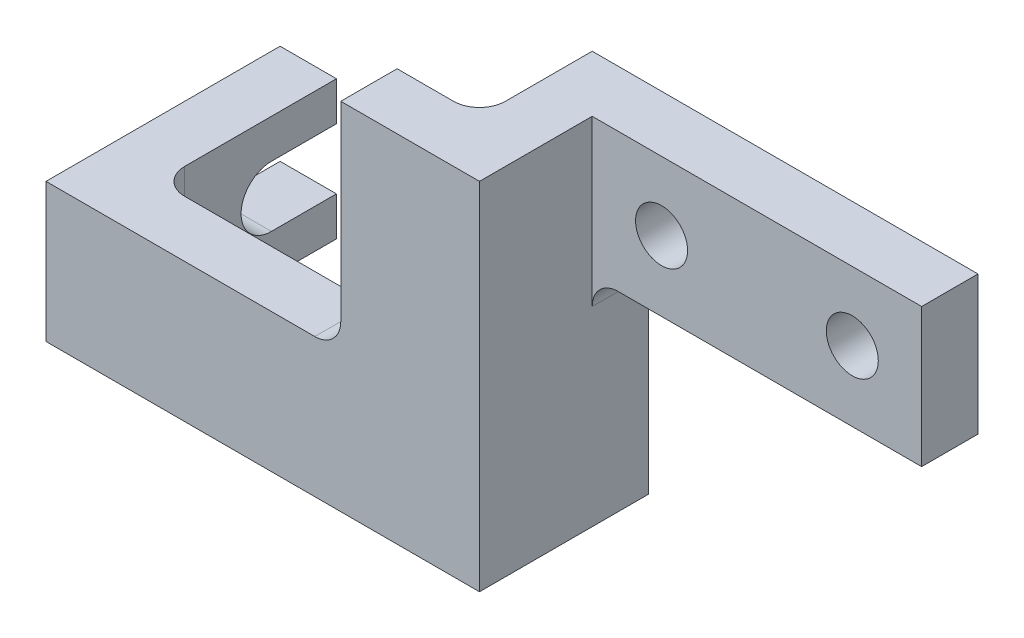
ISO-10303-21;
HEADER;
FILE_DESCRIPTION(('STEP AP214'),'2;1');
FILE_NAME('part.step','',(''),(''),'','','');
FILE_SCHEMA(('AUTOMOTIVE_DESIGN { 1 0 10303 214 1 1 1 1 }'));
ENDSEC;
DATA;
#1=APPLICATION_CONTEXT('core data for automotive mechanical design processes');
#2=APPLICATION_PROTOCOL_DEFINITION('international standard','automotive_design',2000,#1);
#3=PRODUCT_CONTEXT('',#1,'mechanical');
#4=PRODUCT('Part','Part','',(#3));
#5=PRODUCT_RELATED_PRODUCT_CATEGORY('part','',(#4));
#6=PRODUCT_DEFINITION_FORMATION('','',#4);
#7=PRODUCT_DEFINITION_CONTEXT('part definition',#1,'design');
#8=PRODUCT_DEFINITION('design','',#6,#7);
#9=PRODUCT_DEFINITION_SHAPE('','',#8);
#10=(LENGTH_UNIT() NAMED_UNIT(*) SI_UNIT(.MILLI.,.METRE.));
#11=(NAMED_UNIT(*) PLANE_ANGLE_UNIT() SI_UNIT($,.RADIAN.));
#12=(NAMED_UNIT(*) SI_UNIT($,.STERADIAN.) SOLID_ANGLE_UNIT());
#13=UNCERTAINTY_MEASURE_WITH_UNIT(LENGTH_MEASURE(1.E-05),#10,'distance_accuracy_value','');
#14=(GEOMETRIC_REPRESENTATION_CONTEXT(3) GLOBAL_UNCERTAINTY_ASSIGNED_CONTEXT((#13)) GLOBAL_UNIT_ASSIGNED_CONTEXT((#10,
#11,#12)) REPRESENTATION_CONTEXT('',''));
#15=CARTESIAN_POINT('',(0.,0.,0.));
#16=DIRECTION('',(0.,0.,1.));
#17=DIRECTION('',(1.,0.,0.));
#18=AXIS2_PLACEMENT_3D('',#15,#16,#17);
#19=CARTESIAN_POINT('',(0.,0.,-41.));
#20=DIRECTION('',(0.,0.,1.));
#21=DIRECTION('',(1.,0.,0.));
#22=AXIS2_PLACEMENT_3D('',#19,#20,#21);
#23=PLANE('',#22);
#24=DIRECTION('',(0.,-1.,0.));
#25=VECTOR('',#24,1.);
#26=CARTESIAN_POINT('',(13.,0.,-41.));
#27=LINE('',#26,#25);
#28=CARTESIAN_POINT('',(13.,32.,-41.));
#29=VERTEX_POINT('',#28);
#30=CARTESIAN_POINT('',(13.,23.,-41.));
#31=VERTEX_POINT('',#30);
#32=EDGE_CURVE('E352',#29,#31,#27,.T.);
#33=ORIENTED_EDGE('',*,*,#32,.T.);
#34=DIRECTION('',(-1.,0.,0.));
#35=VECTOR('',#34,1.);
#36=CARTESIAN_POINT('',(13.,23.,-41.));
#37=LINE('',#36,#35);
#38=CARTESIAN_POINT('',(0.,23.,-41.));
#39=VERTEX_POINT('',#38);
#40=EDGE_CURVE('E356',#31,#39,#37,.T.);
#41=ORIENTED_EDGE('',*,*,#40,.T.);
#42=DIRECTION('',(0.,1.,0.));
#43=VECTOR('',#42,1.);
#44=CARTESIAN_POINT('',(0.,32.,-41.));
#45=LINE('',#44,#43);
#46=CARTESIAN_POINT('',(0.,32.,-41.));
#47=VERTEX_POINT('',#46);
#48=EDGE_CURVE('E249',#39,#47,#45,.T.);
#49=ORIENTED_EDGE('',*,*,#48,.T.);
#50=DIRECTION('',(1.,0.,0.));
#51=VECTOR('',#50,1.);
#52=CARTESIAN_POINT('',(13.,32.,-41.));
#53=LINE('',#52,#51);
#54=EDGE_CURVE('E248',#47,#29,#53,.T.);
#55=ORIENTED_EDGE('',*,*,#54,.T.);
#56=EDGE_LOOP('',(#33,#41,#49,#55));
#57=FACE_BOUND('',#56,.T.);
#58=ADVANCED_FACE('F50',(#57),#23,.F.);
#59=CARTESIAN_POINT('',(62.,38.,0.));
#60=DIRECTION('',(0.,0.,1.));
#61=DIRECTION('',(1.,0.,0.));
#62=AXIS2_PLACEMENT_3D('',#59,#60,#61);
#63=PLANE('',#62);
#64=DIRECTION('',(0.,-1.,0.));
#65=VECTOR('',#64,1.);
#66=CARTESIAN_POINT('',(81.,82.,0.));
#67=LINE('',#66,#65);
#68=CARTESIAN_POINT('',(81.,82.,0.));
#69=VERTEX_POINT('',#68);
#70=CARTESIAN_POINT('',(81.,0.,0.));
#71=VERTEX_POINT('',#70);
#72=EDGE_CURVE('E275',#69,#71,#67,.T.);
#73=ORIENTED_EDGE('',*,*,#72,.T.);
#74=DIRECTION('',(1.,0.,0.));
#75=VECTOR('',#74,1.);
#76=CARTESIAN_POINT('',(0.,0.,0.));
#77=LINE('',#76,#75);
#78=CARTESIAN_POINT('',(19.,0.,0.));
#79=VERTEX_POINT('',#78);
#80=EDGE_CURVE('E298',#79,#71,#77,.T.);
#81=ORIENTED_EDGE('',*,*,#80,.F.);
#82=DIRECTION('',(0.,-1.,0.));
#83=VECTOR('',#82,1.);
#84=CARTESIAN_POINT('',(19.,82.,0.));
#85=LINE('',#84,#83);
#86=CARTESIAN_POINT('',(19.,32.,0.));
#87=VERTEX_POINT('',#86);
#88=EDGE_CURVE('E11',#87,#79,#85,.T.);
#89=ORIENTED_EDGE('',*,*,#88,.F.);
#90=DIRECTION('',(-1.,0.,0.));
#91=VECTOR('',#90,1.);
#92=CARTESIAN_POINT('',(62.,32.,0.));
#93=LINE('',#92,#91);
#94=CARTESIAN_POINT('',(62.,32.,0.));
#95=VERTEX_POINT('',#94);
#96=EDGE_CURVE('E296',#95,#87,#93,.T.);
#97=ORIENTED_EDGE('',*,*,#96,.F.);
#98=CARTESIAN_POINT('',(62.,38.,0.));
#99=DIRECTION('',(0.,0.,-1.));
#100=DIRECTION('',(1.,0.,0.));
#101=AXIS2_PLACEMENT_3D('',#98,#99,#100);
#102=CIRCLE('',#101,6.);
#103=CARTESIAN_POINT('',(68.,38.,0.));
#104=VERTEX_POINT('',#103);
#105=EDGE_CURVE('E317',#104,#95,#102,.T.);
#106=ORIENTED_EDGE('',*,*,#105,.F.);
#107=DIRECTION('',(0.,-1.,0.));
#108=VECTOR('',#107,1.);
#109=CARTESIAN_POINT('',(68.,82.,0.));
#110=LINE('',#109,#108);
#111=CARTESIAN_POINT('',(68.,82.,0.));
#112=VERTEX_POINT('',#111);
#113=EDGE_CURVE('E313',#112,#104,#110,.T.);
#114=ORIENTED_EDGE('',*,*,#113,.F.);
#115=DIRECTION('',(-1.,0.,0.));
#116=VECTOR('',#115,1.);
#117=CARTESIAN_POINT('',(100.,82.,0.));
#118=LINE('',#117,#116);
#119=EDGE_CURVE('E315',#69,#112,#118,.T.);
#120=ORIENTED_EDGE('',*,*,#119,.F.);
#121=EDGE_LOOP('',(#73,#81,#89,#97,#106,#114,#120));
#122=FACE_BOUND('',#121,.T.);
#123=ADVANCED_FACE('F331',(#122),#63,.F.);
#124=CARTESIAN_POINT('',(0.,32.,13.));
#125=DIRECTION('',(1.,0.,0.));
#126=DIRECTION('',(0.,0.,-1.));
#127=AXIS2_PLACEMENT_3D('',#124,#125,#126);
#128=PLANE('',#127);
#129=ORIENTED_EDGE('',*,*,#48,.F.);
#130=DIRECTION('',(0.,0.,-1.));
#131=VECTOR('',#130,1.);
#132=CARTESIAN_POINT('',(0.,23.,-26.));
#133=LINE('',#132,#131);
#134=CARTESIAN_POINT('',(0.,23.,-26.));
#135=VERTEX_POINT('',#134);
#136=EDGE_CURVE('E358',#135,#39,#133,.T.);
#137=ORIENTED_EDGE('',*,*,#136,.F.);
#138=CARTESIAN_POINT('',(0.,16.,-26.));
#139=DIRECTION('',(-1.,0.,0.));
#140=DIRECTION('',(0.,0.,1.));
#141=AXIS2_PLACEMENT_3D('',#138,#139,#140);
#142=CIRCLE('',#141,7.);
#143=CARTESIAN_POINT('',(0.,9.,-26.));
#144=VERTEX_POINT('',#143);
#145=EDGE_CURVE('E377',#144,#135,#142,.T.);
#146=ORIENTED_EDGE('',*,*,#145,.F.);
#147=DIRECTION('',(0.,0.,1.));
#148=VECTOR('',#147,1.);
#149=CARTESIAN_POINT('',(0.,9.,-41.));
#150=LINE('',#149,#148);
#151=CARTESIAN_POINT('',(0.,9.,-41.));
#152=VERTEX_POINT('',#151);
#153=EDGE_CURVE('E250',#152,#144,#150,.T.);
#154=ORIENTED_EDGE('',*,*,#153,.F.);
#155=CARTESIAN_POINT('',(0.,0.,-41.));
#156=VERTEX_POINT('',#155);
#157=EDGE_CURVE('E242',#156,#152,#45,.T.);
#158=ORIENTED_EDGE('',*,*,#157,.F.);
#159=DIRECTION('',(0.,0.,-1.));
#160=VECTOR('',#159,1.);
#161=CARTESIAN_POINT('',(0.,0.,13.));
#162=LINE('',#161,#160);
#163=CARTESIAN_POINT('',(0.,0.,13.));
#164=VERTEX_POINT('',#163);
#165=EDGE_CURVE('E54',#164,#156,#162,.T.);
#166=ORIENTED_EDGE('',*,*,#165,.F.);
#167=DIRECTION('',(0.,-1.,0.));
#168=VECTOR('',#167,1.);
#169=CARTESIAN_POINT('',(0.,32.,13.));
#170=LINE('',#169,#168);
#171=CARTESIAN_POINT('',(0.,32.,13.));
#172=VERTEX_POINT('',#171);
#173=EDGE_CURVE('E241',#172,#164,#170,.T.);
#174=ORIENTED_EDGE('',*,*,#173,.F.);
#175=DIRECTION('',(0.,0.,-1.));
#176=VECTOR('',#175,1.);
#177=CARTESIAN_POINT('',(0.,32.,13.));
#178=LINE('',#177,#176);
#179=EDGE_CURVE('E307',#172,#47,#178,.T.);
#180=ORIENTED_EDGE('',*,*,#179,.T.);
#181=EDGE_LOOP('',(#129,#137,#146,#154,#158,#166,#174,#180));
#182=FACE_BOUND('',#181,.T.);
#183=ADVANCED_FACE('F47',(#182),#128,.F.);
#184=CARTESIAN_POINT('',(0.,0.,13.));
#185=DIRECTION('',(0.,1.,0.));
#186=DIRECTION('',(0.,0.,1.));
#187=AXIS2_PLACEMENT_3D('',#184,#185,#186);
#188=PLANE('',#187);
#189=ORIENTED_EDGE('',*,*,#165,.T.);
#190=DIRECTION('',(-1.,0.,0.));
#191=VECTOR('',#190,1.);
#192=CARTESIAN_POINT('',(0.,0.,-41.));
#193=LINE('',#192,#191);
#194=CARTESIAN_POINT('',(13.,0.,-41.));
#195=VERTEX_POINT('',#194);
#196=EDGE_CURVE('E233',#195,#156,#193,.T.);
#197=ORIENTED_EDGE('',*,*,#196,.F.);
#198=DIRECTION('',(0.,0.,1.));
#199=VECTOR('',#198,1.);
#200=CARTESIAN_POINT('',(13.,0.,0.));
#201=LINE('',#200,#199);
#202=CARTESIAN_POINT('',(13.,0.,-6.00000000000004));
#203=VERTEX_POINT('',#202);
#204=EDGE_CURVE('E293',#195,#203,#201,.T.);
#205=ORIENTED_EDGE('',*,*,#204,.T.);
#206=CARTESIAN_POINT('',(19.,0.,-6.));
#207=DIRECTION('',(0.,-1.,0.));
#208=DIRECTION('',(0.,0.,-1.));
#209=AXIS2_PLACEMENT_3D('',#206,#207,#208);
#210=CIRCLE('',#209,6.);
#211=EDGE_CURVE('E281',#79,#203,#210,.T.);
#212=ORIENTED_EDGE('',*,*,#211,.F.);
#213=ORIENTED_EDGE('',*,*,#80,.T.);
#214=CARTESIAN_POINT('',(81.,0.,-6.));
#215=DIRECTION('',(0.,-1.,0.));
#216=DIRECTION('',(0.,0.,-1.));
#217=AXIS2_PLACEMENT_3D('',#214,#215,#216);
#218=CIRCLE('',#217,6.);
#219=CARTESIAN_POINT('',(87.,0.,-6.00000000000004));
#220=VERTEX_POINT('',#219);
#221=EDGE_CURVE('E261',#71,#220,#218,.F.);
#222=ORIENTED_EDGE('',*,*,#221,.T.);
#223=DIRECTION('',(0.,0.,-1.));
#224=VECTOR('',#223,1.);
#225=CARTESIAN_POINT('',(87.,0.,0.));
#226=LINE('',#225,#224);
#227=CARTESIAN_POINT('',(87.,0.,-26.));
#228=VERTEX_POINT('',#227);
#229=EDGE_CURVE('E273',#220,#228,#226,.T.);
#230=ORIENTED_EDGE('',*,*,#229,.T.);
#231=DIRECTION('',(1.,0.,0.));
#232=VECTOR('',#231,1.);
#233=CARTESIAN_POINT('',(0.,0.,-26.));
#234=LINE('',#233,#232);
#235=CARTESIAN_POINT('',(100.,0.,-26.));
#236=VERTEX_POINT('',#235);
#237=EDGE_CURVE('E270',#228,#236,#234,.T.);
#238=ORIENTED_EDGE('',*,*,#237,.T.);
#239=DIRECTION('',(0.,0.,-1.));
#240=VECTOR('',#239,1.);
#241=CARTESIAN_POINT('',(100.,0.,13.));
#242=LINE('',#241,#240);
#243=CARTESIAN_POINT('',(100.,0.,13.));
#244=VERTEX_POINT('',#243);
#245=EDGE_CURVE('E216',#244,#236,#242,.T.);
#246=ORIENTED_EDGE('',*,*,#245,.F.);
#247=DIRECTION('',(1.,0.,0.));
#248=VECTOR('',#247,1.);
#249=CARTESIAN_POINT('',(0.,0.,13.));
#250=LINE('',#249,#248);
#251=EDGE_CURVE('E234',#164,#244,#250,.T.);
#252=ORIENTED_EDGE('',*,*,#251,.F.);
#253=EDGE_LOOP('',(#189,#197,#205,#212,#213,#222,#230,#238,#246,#252));
#254=FACE_BOUND('',#253,.T.);
#255=ADVANCED_FACE('F229',(#254),#188,.F.);
#256=CARTESIAN_POINT('',(100.,0.,13.));
#257=DIRECTION('',(-1.,0.,0.));
#258=DIRECTION('',(0.,0.,1.));
#259=AXIS2_PLACEMENT_3D('',#256,#257,#258);
#260=PLANE('',#259);
#261=DIRECTION('',(0.,-1.,0.));
#262=VECTOR('',#261,1.);
#263=CARTESIAN_POINT('',(100.,82.,-26.));
#264=LINE('',#263,#262);
#265=CARTESIAN_POINT('',(100.,44.,-26.));
#266=VERTEX_POINT('',#265);
#267=EDGE_CURVE('E278',#266,#236,#264,.T.);
#268=ORIENTED_EDGE('',*,*,#267,.F.);
#269=DIRECTION('',(0.,0.,-1.));
#270=VECTOR('',#269,1.);
#271=CARTESIAN_POINT('',(100.,44.,-13.));
#272=LINE('',#271,#270);
#273=CARTESIAN_POINT('',(100.,44.,-13.));
#274=VERTEX_POINT('',#273);
#275=EDGE_CURVE('E215',#274,#266,#272,.T.);
#276=ORIENTED_EDGE('',*,*,#275,.F.);
#277=DIRECTION('',(0.,1.,0.));
#278=VECTOR('',#277,1.);
#279=CARTESIAN_POINT('',(100.,82.,-13.));
#280=LINE('',#279,#278);
#281=CARTESIAN_POINT('',(100.,82.,-13.));
#282=VERTEX_POINT('',#281);
#283=EDGE_CURVE('E193',#274,#282,#280,.T.);
#284=ORIENTED_EDGE('',*,*,#283,.T.);
#285=DIRECTION('',(0.,0.,-1.));
#286=VECTOR('',#285,1.);
#287=CARTESIAN_POINT('',(100.,82.,13.));
#288=LINE('',#287,#286);
#289=CARTESIAN_POINT('',(100.,82.,13.));
#290=VERTEX_POINT('',#289);
#291=EDGE_CURVE('E208',#290,#282,#288,.T.);
#292=ORIENTED_EDGE('',*,*,#291,.F.);
#293=DIRECTION('',(0.,1.,0.));
#294=VECTOR('',#293,1.);
#295=CARTESIAN_POINT('',(100.,0.,13.));
#296=LINE('',#295,#294);
#297=EDGE_CURVE('E297',#244,#290,#296,.T.);
#298=ORIENTED_EDGE('',*,*,#297,.F.);
#299=ORIENTED_EDGE('',*,*,#245,.T.);
#300=EDGE_LOOP('',(#268,#276,#284,#292,#298,#299));
#301=FACE_BOUND('',#300,.T.);
#302=ADVANCED_FACE('F206',(#301),#260,.F.);
#303=CARTESIAN_POINT('',(100.,82.,13.));
#304=DIRECTION('',(0.,-1.,0.));
#305=DIRECTION('',(0.,0.,-1.));
#306=AXIS2_PLACEMENT_3D('',#303,#304,#305);
#307=PLANE('',#306);
#308=ORIENTED_EDGE('',*,*,#291,.T.);
#309=DIRECTION('',(1.,0.,0.));
#310=VECTOR('',#309,1.);
#311=CARTESIAN_POINT('',(100.,82.,-13.));
#312=LINE('',#311,#310);
#313=CARTESIAN_POINT('',(176.,82.,-13.));
#314=VERTEX_POINT('',#313);
#315=EDGE_CURVE('E192',#282,#314,#312,.T.);
#316=ORIENTED_EDGE('',*,*,#315,.T.);
#317=DIRECTION('',(0.,0.,-1.));
#318=VECTOR('',#317,1.);
#319=CARTESIAN_POINT('',(176.,82.,-13.));
#320=LINE('',#319,#318);
#321=CARTESIAN_POINT('',(176.,82.,-26.));
#322=VERTEX_POINT('',#321);
#323=EDGE_CURVE('E379',#314,#322,#320,.T.);
#324=ORIENTED_EDGE('',*,*,#323,.T.);
#325=DIRECTION('',(1.,0.,0.));
#326=VECTOR('',#325,1.);
#327=CARTESIAN_POINT('',(0.,82.,-26.));
#328=LINE('',#327,#326);
#329=CARTESIAN_POINT('',(87.,82.,-26.));
#330=VERTEX_POINT('',#329);
#331=EDGE_CURVE('E268',#330,#322,#328,.T.);
#332=ORIENTED_EDGE('',*,*,#331,.F.);
#333=DIRECTION('',(0.,0.,-1.));
#334=VECTOR('',#333,1.);
#335=CARTESIAN_POINT('',(87.,82.,0.));
#336=LINE('',#335,#334);
#337=CARTESIAN_POINT('',(87.,82.,-6.00000000000004));
#338=VERTEX_POINT('',#337);
#339=EDGE_CURVE('E267',#338,#330,#336,.T.);
#340=ORIENTED_EDGE('',*,*,#339,.F.);
#341=CARTESIAN_POINT('',(81.,82.,-6.));
#342=DIRECTION('',(0.,-1.,0.));
#343=DIRECTION('',(0.,0.,-1.));
#344=AXIS2_PLACEMENT_3D('',#341,#342,#343);
#345=CIRCLE('',#344,6.);
#346=EDGE_CURVE('E265',#69,#338,#345,.F.);
#347=ORIENTED_EDGE('',*,*,#346,.F.);
#348=ORIENTED_EDGE('',*,*,#119,.T.);
#349=DIRECTION('',(0.,0.,-1.));
#350=VECTOR('',#349,1.);
#351=CARTESIAN_POINT('',(68.,82.,13.));
#352=LINE('',#351,#350);
#353=CARTESIAN_POINT('',(68.,82.,13.));
#354=VERTEX_POINT('',#353);
#355=EDGE_CURVE('E220',#354,#112,#352,.T.);
#356=ORIENTED_EDGE('',*,*,#355,.F.);
#357=DIRECTION('',(-1.,0.,0.));
#358=VECTOR('',#357,1.);
#359=CARTESIAN_POINT('',(100.,82.,13.));
#360=LINE('',#359,#358);
#361=EDGE_CURVE('E219',#290,#354,#360,.T.);
#362=ORIENTED_EDGE('',*,*,#361,.F.);
#363=EDGE_LOOP('',(#308,#316,#324,#332,#340,#347,#348,#356,#362));
#364=FACE_BOUND('',#363,.T.);
#365=ADVANCED_FACE('F211',(#364),#307,.F.);
#366=CARTESIAN_POINT('',(68.,82.,13.));
#367=DIRECTION('',(1.,0.,0.));
#368=DIRECTION('',(0.,0.,-1.));
#369=AXIS2_PLACEMENT_3D('',#366,#367,#368);
#370=PLANE('',#369);
#371=ORIENTED_EDGE('',*,*,#113,.T.);
#372=DIRECTION('',(0.,0.,-1.));
#373=VECTOR('',#372,1.);
#374=CARTESIAN_POINT('',(68.,38.,13.));
#375=LINE('',#374,#373);
#376=CARTESIAN_POINT('',(68.,38.,13.));
#377=VERTEX_POINT('',#376);
#378=EDGE_CURVE('E224',#377,#104,#375,.T.);
#379=ORIENTED_EDGE('',*,*,#378,.F.);
#380=DIRECTION('',(0.,-1.,0.));
#381=VECTOR('',#380,1.);
#382=CARTESIAN_POINT('',(68.,82.,13.));
#383=LINE('',#382,#381);
#384=EDGE_CURVE('E303',#354,#377,#383,.T.);
#385=ORIENTED_EDGE('',*,*,#384,.F.);
#386=ORIENTED_EDGE('',*,*,#355,.T.);
#387=EDGE_LOOP('',(#371,#379,#385,#386));
#388=FACE_BOUND('',#387,.T.);
#389=ADVANCED_FACE('F441',(#388),#370,.F.);
#390=CARTESIAN_POINT('',(62.,38.,13.));
#391=DIRECTION('',(0.,0.,-1.));
#392=DIRECTION('',(-1.,0.,0.));
#393=AXIS2_PLACEMENT_3D('',#390,#391,#392);
#394=CYLINDRICAL_SURFACE('',#393,6.);
#395=ORIENTED_EDGE('',*,*,#105,.T.);
#396=DIRECTION('',(0.,0.,-1.));
#397=VECTOR('',#396,1.);
#398=CARTESIAN_POINT('',(62.,32.,13.));
#399=LINE('',#398,#397);
#400=CARTESIAN_POINT('',(62.,32.,13.));
#401=VERTEX_POINT('',#400);
#402=EDGE_CURVE('E318',#401,#95,#399,.T.);
#403=ORIENTED_EDGE('',*,*,#402,.F.);
#404=CARTESIAN_POINT('',(62.,38.,13.));
#405=DIRECTION('',(0.,0.,-1.));
#406=DIRECTION('',(1.,0.,0.));
#407=AXIS2_PLACEMENT_3D('',#404,#405,#406);
#408=CIRCLE('',#407,6.);
#409=EDGE_CURVE('E304',#377,#401,#408,.T.);
#410=ORIENTED_EDGE('',*,*,#409,.F.);
#411=ORIENTED_EDGE('',*,*,#378,.T.);
#412=EDGE_LOOP('',(#395,#403,#410,#411));
#413=FACE_BOUND('',#412,.T.);
#414=ADVANCED_FACE('F326',(#413),#394,.F.);
#415=CARTESIAN_POINT('',(62.,32.,13.));
#416=DIRECTION('',(0.,-1.,0.));
#417=DIRECTION('',(0.,0.,-1.));
#418=AXIS2_PLACEMENT_3D('',#415,#416,#417);
#419=PLANE('',#418);
#420=DIRECTION('',(0.,0.,-1.));
#421=VECTOR('',#420,1.);
#422=CARTESIAN_POINT('',(13.,32.,0.));
#423=LINE('',#422,#421);
#424=CARTESIAN_POINT('',(13.,32.,-6.00000000000004));
#425=VERTEX_POINT('',#424);
#426=EDGE_CURVE('E255',#425,#29,#423,.T.);
#427=ORIENTED_EDGE('',*,*,#426,.T.);
#428=ORIENTED_EDGE('',*,*,#54,.F.);
#429=ORIENTED_EDGE('',*,*,#179,.F.);
#430=DIRECTION('',(-1.,0.,0.));
#431=VECTOR('',#430,1.);
#432=CARTESIAN_POINT('',(62.,32.,13.));
#433=LINE('',#432,#431);
#434=EDGE_CURVE('E310',#401,#172,#433,.T.);
#435=ORIENTED_EDGE('',*,*,#434,.F.);
#436=ORIENTED_EDGE('',*,*,#402,.T.);
#437=ORIENTED_EDGE('',*,*,#96,.T.);
#438=CARTESIAN_POINT('',(19.,32.,-6.));
#439=DIRECTION('',(0.,-1.,0.));
#440=DIRECTION('',(0.,0.,-1.));
#441=AXIS2_PLACEMENT_3D('',#438,#439,#440);
#442=CIRCLE('',#441,6.);
#443=EDGE_CURVE('E256',#425,#87,#442,.F.);
#444=ORIENTED_EDGE('',*,*,#443,.F.);
#445=EDGE_LOOP('',(#427,#428,#429,#435,#436,#437,#444));
#446=FACE_BOUND('',#445,.T.);
#447=ADVANCED_FACE('F339',(#446),#419,.F.);
#448=CARTESIAN_POINT('',(62.,38.,13.));
#449=DIRECTION('',(0.,0.,1.));
#450=DIRECTION('',(1.,0.,0.));
#451=AXIS2_PLACEMENT_3D('',#448,#449,#450);
#452=PLANE('',#451);
#453=ORIENTED_EDGE('',*,*,#173,.T.);
#454=ORIENTED_EDGE('',*,*,#251,.T.);
#455=ORIENTED_EDGE('',*,*,#297,.T.);
#456=ORIENTED_EDGE('',*,*,#361,.T.);
#457=ORIENTED_EDGE('',*,*,#384,.T.);
#458=ORIENTED_EDGE('',*,*,#409,.T.);
#459=ORIENTED_EDGE('',*,*,#434,.T.);
#460=EDGE_LOOP('',(#453,#454,#455,#456,#457,#458,#459));
#461=FACE_BOUND('',#460,.T.);
#462=ADVANCED_FACE('F433',(#461),#452,.T.);
#463=CARTESIAN_POINT('',(19.,82.,-6.));
#464=DIRECTION('',(0.,-1.,0.));
#465=DIRECTION('',(0.,0.,-1.));
#466=AXIS2_PLACEMENT_3D('',#463,#464,#465);
#467=CYLINDRICAL_SURFACE('',#466,6.);
#468=DIRECTION('',(0.,-1.,0.));
#469=VECTOR('',#468,1.);
#470=CARTESIAN_POINT('',(13.,82.,-6.00000000000004));
#471=LINE('',#470,#469);
#472=EDGE_CURVE('E291',#425,#203,#471,.T.);
#473=ORIENTED_EDGE('',*,*,#472,.F.);
#474=ORIENTED_EDGE('',*,*,#443,.T.);
#475=ORIENTED_EDGE('',*,*,#88,.T.);
#476=ORIENTED_EDGE('',*,*,#211,.T.);
#477=EDGE_LOOP('',(#473,#474,#475,#476));
#478=FACE_BOUND('',#477,.T.);
#479=ADVANCED_FACE('F341',(#478),#467,.F.);
#480=CARTESIAN_POINT('',(13.,82.,0.));
#481=DIRECTION('',(1.,0.,0.));
#482=DIRECTION('',(0.,0.,-1.));
#483=AXIS2_PLACEMENT_3D('',#480,#481,#482);
#484=PLANE('',#483);
#485=DIRECTION('',(0.,0.,-1.));
#486=VECTOR('',#485,1.);
#487=CARTESIAN_POINT('',(13.,23.,-26.));
#488=LINE('',#487,#486);
#489=CARTESIAN_POINT('',(13.,23.,-26.));
#490=VERTEX_POINT('',#489);
#491=EDGE_CURVE('E371',#490,#31,#488,.T.);
#492=ORIENTED_EDGE('',*,*,#491,.T.);
#493=ORIENTED_EDGE('',*,*,#32,.F.);
#494=ORIENTED_EDGE('',*,*,#426,.F.);
#495=ORIENTED_EDGE('',*,*,#472,.T.);
#496=ORIENTED_EDGE('',*,*,#204,.F.);
#497=CARTESIAN_POINT('',(13.,9.,-41.));
#498=VERTEX_POINT('',#497);
#499=EDGE_CURVE('E363',#498,#195,#27,.T.);
#500=ORIENTED_EDGE('',*,*,#499,.F.);
#501=DIRECTION('',(0.,0.,1.));
#502=VECTOR('',#501,1.);
#503=CARTESIAN_POINT('',(13.,9.,-41.));
#504=LINE('',#503,#502);
#505=CARTESIAN_POINT('',(13.,9.,-26.));
#506=VERTEX_POINT('',#505);
#507=EDGE_CURVE('E67',#498,#506,#504,.T.);
#508=ORIENTED_EDGE('',*,*,#507,.T.);
#509=CARTESIAN_POINT('',(13.,16.,-26.));
#510=DIRECTION('',(-1.,0.,0.));
#511=DIRECTION('',(0.,0.,1.));
#512=AXIS2_PLACEMENT_3D('',#509,#510,#511);
#513=CIRCLE('',#512,7.);
#514=EDGE_CURVE('E374',#506,#490,#513,.T.);
#515=ORIENTED_EDGE('',*,*,#514,.T.);
#516=EDGE_LOOP('',(#492,#493,#494,#495,#496,#500,#508,#515));
#517=FACE_BOUND('',#516,.T.);
#518=ADVANCED_FACE('F346',(#517),#484,.T.);
#519=CARTESIAN_POINT('',(0.,82.,-26.));
#520=DIRECTION('',(0.,0.,-1.));
#521=DIRECTION('',(-1.,0.,0.));
#522=AXIS2_PLACEMENT_3D('',#519,#520,#521);
#523=PLANE('',#522);
#524=CARTESIAN_POINT('',(116.,66.1568766824244,-26.));
#525=DIRECTION('',(0.,0.,1.));
#526=DIRECTION('',(1.,0.,0.));
#527=AXIS2_PLACEMENT_3D('',#524,#525,#526);
#528=CIRCLE('',#527,5.99999999999999);
#529=CARTESIAN_POINT('',(122.,66.1568766824244,-26.));
#530=VERTEX_POINT('',#529);
#531=EDGE_CURVE('E706',#530,#530,#528,.T.);
#532=ORIENTED_EDGE('',*,*,#531,.T.);
#533=EDGE_LOOP('',(#532));
#534=FACE_BOUND('',#533,.T.);
#535=CARTESIAN_POINT('',(160.,66.1568766824244,-26.));
#536=DIRECTION('',(0.,0.,1.));
#537=DIRECTION('',(1.,0.,0.));
#538=AXIS2_PLACEMENT_3D('',#535,#536,#537);
#539=CIRCLE('',#538,5.99999999999999);
#540=CARTESIAN_POINT('',(166.,66.1568766824244,-26.));
#541=VERTEX_POINT('',#540);
#542=EDGE_CURVE('E715',#541,#541,#539,.T.);
#543=ORIENTED_EDGE('',*,*,#542,.T.);
#544=EDGE_LOOP('',(#543));
#545=FACE_BOUND('',#544,.T.);
#546=ORIENTED_EDGE('',*,*,#237,.F.);
#547=DIRECTION('',(0.,-1.,0.));
#548=VECTOR('',#547,1.);
#549=CARTESIAN_POINT('',(87.,82.,-26.));
#550=LINE('',#549,#548);
#551=EDGE_CURVE('E285',#330,#228,#550,.T.);
#552=ORIENTED_EDGE('',*,*,#551,.F.);
#553=ORIENTED_EDGE('',*,*,#331,.T.);
#554=DIRECTION('',(0.,-1.,0.));
#555=VECTOR('',#554,1.);
#556=CARTESIAN_POINT('',(176.,82.,-26.));
#557=LINE('',#556,#555);
#558=CARTESIAN_POINT('',(176.,50.,-26.));
#559=VERTEX_POINT('',#558);
#560=EDGE_CURVE('E717',#322,#559,#557,.T.);
#561=ORIENTED_EDGE('',*,*,#560,.T.);
#562=DIRECTION('',(-1.,0.,0.));
#563=VECTOR('',#562,1.);
#564=CARTESIAN_POINT('',(176.,50.,-26.));
#565=LINE('',#564,#563);
#566=CARTESIAN_POINT('',(106.,50.,-26.));
#567=VERTEX_POINT('',#566);
#568=EDGE_CURVE('E725',#559,#567,#565,.T.);
#569=ORIENTED_EDGE('',*,*,#568,.T.);
#570=CARTESIAN_POINT('',(106.,44.,-26.));
#571=DIRECTION('',(0.,0.,1.));
#572=DIRECTION('',(1.,0.,0.));
#573=AXIS2_PLACEMENT_3D('',#570,#571,#572);
#574=CIRCLE('',#573,6.);
#575=EDGE_CURVE('E65',#567,#266,#574,.T.);
#576=ORIENTED_EDGE('',*,*,#575,.T.);
#577=ORIENTED_EDGE('',*,*,#267,.T.);
#578=EDGE_LOOP('',(#546,#552,#553,#561,#569,#576,#577));
#579=FACE_BOUND('',#578,.T.);
#580=ADVANCED_FACE('F428',(#534,#545,#579),#523,.T.);
#581=CARTESIAN_POINT('',(87.,82.,0.));
#582=DIRECTION('',(-1.,0.,0.));
#583=DIRECTION('',(0.,0.,1.));
#584=AXIS2_PLACEMENT_3D('',#581,#582,#583);
#585=PLANE('',#584);
#586=ORIENTED_EDGE('',*,*,#229,.F.);
#587=DIRECTION('',(0.,-1.,0.));
#588=VECTOR('',#587,1.);
#589=CARTESIAN_POINT('',(87.,82.,-6.00000000000004));
#590=LINE('',#589,#588);
#591=EDGE_CURVE('E282',#338,#220,#590,.T.);
#592=ORIENTED_EDGE('',*,*,#591,.F.);
#593=ORIENTED_EDGE('',*,*,#339,.T.);
#594=ORIENTED_EDGE('',*,*,#551,.T.);
#595=EDGE_LOOP('',(#586,#592,#593,#594));
#596=FACE_BOUND('',#595,.T.);
#597=ADVANCED_FACE('F416',(#596),#585,.T.);
#598=CARTESIAN_POINT('',(81.,82.,-6.));
#599=DIRECTION('',(0.,-1.,0.));
#600=DIRECTION('',(0.,0.,-1.));
#601=AXIS2_PLACEMENT_3D('',#598,#599,#600);
#602=CYLINDRICAL_SURFACE('',#601,6.);
#603=ORIENTED_EDGE('',*,*,#221,.F.);
#604=ORIENTED_EDGE('',*,*,#72,.F.);
#605=ORIENTED_EDGE('',*,*,#346,.T.);
#606=ORIENTED_EDGE('',*,*,#591,.T.);
#607=EDGE_LOOP('',(#603,#604,#605,#606));
#608=FACE_BOUND('',#607,.T.);
#609=ADVANCED_FACE('F414',(#608),#602,.F.);
#610=ORIENTED_EDGE('',*,*,#157,.T.);
#611=DIRECTION('',(-1.,0.,0.));
#612=VECTOR('',#611,1.);
#613=CARTESIAN_POINT('',(13.,9.,-41.));
#614=LINE('',#613,#612);
#615=EDGE_CURVE('E369',#498,#152,#614,.T.);
#616=ORIENTED_EDGE('',*,*,#615,.F.);
#617=ORIENTED_EDGE('',*,*,#499,.T.);
#618=ORIENTED_EDGE('',*,*,#196,.T.);
#619=EDGE_LOOP('',(#610,#616,#617,#618));
#620=FACE_BOUND('',#619,.T.);
#621=ADVANCED_FACE('F375',(#620),#23,.F.);
#622=CARTESIAN_POINT('',(13.,23.,-26.));
#623=DIRECTION('',(0.,1.,0.));
#624=DIRECTION('',(0.,0.,1.));
#625=AXIS2_PLACEMENT_3D('',#622,#623,#624);
#626=PLANE('',#625);
#627=ORIENTED_EDGE('',*,*,#136,.T.);
#628=ORIENTED_EDGE('',*,*,#40,.F.);
#629=ORIENTED_EDGE('',*,*,#491,.F.);
#630=DIRECTION('',(-1.,0.,0.));
#631=VECTOR('',#630,1.);
#632=CARTESIAN_POINT('',(13.,23.,-26.));
#633=LINE('',#632,#631);
#634=EDGE_CURVE('E365',#490,#135,#633,.T.);
#635=ORIENTED_EDGE('',*,*,#634,.T.);
#636=EDGE_LOOP('',(#627,#628,#629,#635));
#637=FACE_BOUND('',#636,.T.);
#638=ADVANCED_FACE('F396',(#637),#626,.F.);
#639=CARTESIAN_POINT('',(13.,16.,-26.));
#640=DIRECTION('',(-1.,0.,0.));
#641=DIRECTION('',(0.,0.,1.));
#642=AXIS2_PLACEMENT_3D('',#639,#640,#641);
#643=CYLINDRICAL_SURFACE('',#642,7.);
#644=ORIENTED_EDGE('',*,*,#145,.T.);
#645=ORIENTED_EDGE('',*,*,#634,.F.);
#646=ORIENTED_EDGE('',*,*,#514,.F.);
#647=DIRECTION('',(-1.,0.,0.));
#648=VECTOR('',#647,1.);
#649=CARTESIAN_POINT('',(13.,9.,-26.));
#650=LINE('',#649,#648);
#651=EDGE_CURVE('E364',#506,#144,#650,.T.);
#652=ORIENTED_EDGE('',*,*,#651,.T.);
#653=EDGE_LOOP('',(#644,#645,#646,#652));
#654=FACE_BOUND('',#653,.T.);
#655=ADVANCED_FACE('F387',(#654),#643,.F.);
#656=CARTESIAN_POINT('',(13.,9.,-41.));
#657=DIRECTION('',(0.,-1.,0.));
#658=DIRECTION('',(0.,0.,-1.));
#659=AXIS2_PLACEMENT_3D('',#656,#657,#658);
#660=PLANE('',#659);
#661=ORIENTED_EDGE('',*,*,#153,.T.);
#662=ORIENTED_EDGE('',*,*,#651,.F.);
#663=ORIENTED_EDGE('',*,*,#507,.F.);
#664=ORIENTED_EDGE('',*,*,#615,.T.);
#665=EDGE_LOOP('',(#661,#662,#663,#664));
#666=FACE_BOUND('',#665,.T.);
#667=ADVANCED_FACE('F390',(#666),#660,.F.);
#668=CARTESIAN_POINT('',(106.,44.,-13.));
#669=DIRECTION('',(0.,0.,-1.));
#670=DIRECTION('',(-1.,0.,0.));
#671=AXIS2_PLACEMENT_3D('',#668,#669,#670);
#672=CYLINDRICAL_SURFACE('',#671,6.);
#673=ORIENTED_EDGE('',*,*,#575,.F.);
#674=DIRECTION('',(0.,0.,-1.));
#675=VECTOR('',#674,1.);
#676=CARTESIAN_POINT('',(106.,50.,-13.));
#677=LINE('',#676,#675);
#678=CARTESIAN_POINT('',(106.,50.,-13.));
#679=VERTEX_POINT('',#678);
#680=EDGE_CURVE('E734',#679,#567,#677,.T.);
#681=ORIENTED_EDGE('',*,*,#680,.F.);
#682=CARTESIAN_POINT('',(106.,44.,-13.));
#683=DIRECTION('',(0.,0.,1.));
#684=DIRECTION('',(1.,0.,0.));
#685=AXIS2_PLACEMENT_3D('',#682,#683,#684);
#686=CIRCLE('',#685,6.);
#687=EDGE_CURVE('E726',#679,#274,#686,.T.);
#688=ORIENTED_EDGE('',*,*,#687,.T.);
#689=ORIENTED_EDGE('',*,*,#275,.T.);
#690=EDGE_LOOP('',(#673,#681,#688,#689));
#691=FACE_BOUND('',#690,.T.);
#692=ADVANCED_FACE('F386',(#691),#672,.F.);
#693=CARTESIAN_POINT('',(176.,50.,-13.));
#694=DIRECTION('',(0.,-1.,0.));
#695=DIRECTION('',(0.,0.,-1.));
#696=AXIS2_PLACEMENT_3D('',#693,#694,#695);
#697=PLANE('',#696);
#698=ORIENTED_EDGE('',*,*,#568,.F.);
#699=DIRECTION('',(0.,0.,-1.));
#700=VECTOR('',#699,1.);
#701=CARTESIAN_POINT('',(176.,50.,-13.));
#702=LINE('',#701,#700);
#703=CARTESIAN_POINT('',(176.,50.,-13.));
#704=VERTEX_POINT('',#703);
#705=EDGE_CURVE('E731',#704,#559,#702,.T.);
#706=ORIENTED_EDGE('',*,*,#705,.F.);
#707=DIRECTION('',(-1.,0.,0.));
#708=VECTOR('',#707,1.);
#709=CARTESIAN_POINT('',(176.,50.,-13.));
#710=LINE('',#709,#708);
#711=EDGE_CURVE('E733',#704,#679,#710,.T.);
#712=ORIENTED_EDGE('',*,*,#711,.T.);
#713=ORIENTED_EDGE('',*,*,#680,.T.);
#714=EDGE_LOOP('',(#698,#706,#712,#713));
#715=FACE_BOUND('',#714,.T.);
#716=ADVANCED_FACE('F397',(#715),#697,.T.);
#717=CARTESIAN_POINT('',(176.,82.,-13.));
#718=DIRECTION('',(1.,0.,0.));
#719=DIRECTION('',(0.,0.,-1.));
#720=AXIS2_PLACEMENT_3D('',#717,#718,#719);
#721=PLANE('',#720);
#722=ORIENTED_EDGE('',*,*,#560,.F.);
#723=ORIENTED_EDGE('',*,*,#323,.F.);
#724=DIRECTION('',(0.,-1.,0.));
#725=VECTOR('',#724,1.);
#726=CARTESIAN_POINT('',(176.,82.,-13.));
#727=LINE('',#726,#725);
#728=EDGE_CURVE('E198',#314,#704,#727,.T.);
#729=ORIENTED_EDGE('',*,*,#728,.T.);
#730=ORIENTED_EDGE('',*,*,#705,.T.);
#731=EDGE_LOOP('',(#722,#723,#729,#730));
#732=FACE_BOUND('',#731,.T.);
#733=ADVANCED_FACE('F547',(#732),#721,.T.);
#734=CARTESIAN_POINT('',(106.,44.,-13.));
#735=DIRECTION('',(0.,0.,1.));
#736=DIRECTION('',(1.,0.,0.));
#737=AXIS2_PLACEMENT_3D('',#734,#735,#736);
#738=PLANE('',#737);
#739=CARTESIAN_POINT('',(116.,66.1568766824244,-13.));
#740=DIRECTION('',(0.,0.,1.));
#741=DIRECTION('',(1.,0.,0.));
#742=AXIS2_PLACEMENT_3D('',#739,#740,#741);
#743=CIRCLE('',#742,5.99999999999999);
#744=CARTESIAN_POINT('',(122.,66.1568766824244,-13.));
#745=VERTEX_POINT('',#744);
#746=EDGE_CURVE('E723',#745,#745,#743,.T.);
#747=ORIENTED_EDGE('',*,*,#746,.F.);
#748=EDGE_LOOP('',(#747));
#749=FACE_BOUND('',#748,.T.);
#750=CARTESIAN_POINT('',(160.,66.1568766824244,-13.));
#751=DIRECTION('',(0.,0.,1.));
#752=DIRECTION('',(1.,0.,0.));
#753=AXIS2_PLACEMENT_3D('',#750,#751,#752);
#754=CIRCLE('',#753,5.99999999999999);
#755=CARTESIAN_POINT('',(166.,66.1568766824244,-13.));
#756=VERTEX_POINT('',#755);
#757=EDGE_CURVE('E738',#756,#756,#754,.T.);
#758=ORIENTED_EDGE('',*,*,#757,.F.);
#759=EDGE_LOOP('',(#758));
#760=FACE_BOUND('',#759,.T.);
#761=ORIENTED_EDGE('',*,*,#283,.F.);
#762=ORIENTED_EDGE('',*,*,#687,.F.);
#763=ORIENTED_EDGE('',*,*,#711,.F.);
#764=ORIENTED_EDGE('',*,*,#728,.F.);
#765=ORIENTED_EDGE('',*,*,#315,.F.);
#766=EDGE_LOOP('',(#761,#762,#763,#764,#765));
#767=FACE_BOUND('',#766,.T.);
#768=ADVANCED_FACE('F194',(#749,#760,#767),#738,.T.);
#769=CARTESIAN_POINT('',(160.,66.1568766824244,-26.));
#770=DIRECTION('',(0.,0.,1.));
#771=DIRECTION('',(1.,0.,0.));
#772=AXIS2_PLACEMENT_3D('',#769,#770,#771);
#773=CYLINDRICAL_SURFACE('',#772,5.99999999999999);
#774=CARTESIAN_POINT('',(166.,66.1568766824244,-26.));
#775=CARTESIAN_POINT('',(166.,66.1568766824244,-25.8645833333333));
#776=CARTESIAN_POINT('',(166.,66.1568766824244,-25.7291666666667));
#777=CARTESIAN_POINT('',(166.,66.1568766824244,-25.4583333333333));
#778=CARTESIAN_POINT('',(166.,66.1568766824244,-25.3229166666667));
#779=CARTESIAN_POINT('',(166.,66.1568766824244,-25.0520833333333));
#780=CARTESIAN_POINT('',(166.,66.1568766824244,-24.9166666666667));
#781=CARTESIAN_POINT('',(166.,66.1568766824244,-24.6458333333333));
#782=CARTESIAN_POINT('',(166.,66.1568766824244,-24.5104166666667));
#783=CARTESIAN_POINT('',(166.,66.1568766824244,-24.2395833333333));
#784=CARTESIAN_POINT('',(166.,66.1568766824244,-24.1041666666667));
#785=CARTESIAN_POINT('',(166.,66.1568766824244,-23.8333333333333));
#786=CARTESIAN_POINT('',(166.,66.1568766824244,-23.6979166666667));
#787=CARTESIAN_POINT('',(166.,66.1568766824244,-23.4270833333333));
#788=CARTESIAN_POINT('',(166.,66.1568766824244,-23.2916666666667));
#789=CARTESIAN_POINT('',(166.,66.1568766824244,-23.0208333333333));
#790=CARTESIAN_POINT('',(166.,66.1568766824244,-22.8854166666667));
#791=CARTESIAN_POINT('',(166.,66.1568766824244,-22.6145833333333));
#792=CARTESIAN_POINT('',(166.,66.1568766824244,-22.4791666666667));
#793=CARTESIAN_POINT('',(166.,66.1568766824244,-22.2083333333333));
#794=CARTESIAN_POINT('',(166.,66.1568766824244,-22.0729166666667));
#795=CARTESIAN_POINT('',(166.,66.1568766824244,-21.8020833333333));
#796=CARTESIAN_POINT('',(166.,66.1568766824244,-21.6666666666667));
#797=CARTESIAN_POINT('',(166.,66.1568766824244,-21.3958333333333));
#798=CARTESIAN_POINT('',(166.,66.1568766824244,-21.2604166666667));
#799=CARTESIAN_POINT('',(166.,66.1568766824244,-20.9895833333333));
#800=CARTESIAN_POINT('',(166.,66.1568766824244,-20.8541666666667));
#801=CARTESIAN_POINT('',(166.,66.1568766824244,-20.5833333333333));
#802=CARTESIAN_POINT('',(166.,66.1568766824244,-20.4479166666667));
#803=CARTESIAN_POINT('',(166.,66.1568766824244,-20.1770833333333));
#804=CARTESIAN_POINT('',(166.,66.1568766824244,-20.0416666666667));
#805=CARTESIAN_POINT('',(166.,66.1568766824244,-19.7708333333333));
#806=CARTESIAN_POINT('',(166.,66.1568766824244,-19.6354166666667));
#807=CARTESIAN_POINT('',(166.,66.1568766824244,-19.3645833333333));
#808=CARTESIAN_POINT('',(166.,66.1568766824244,-19.2291666666667));
#809=CARTESIAN_POINT('',(166.,66.1568766824244,-18.9583333333333));
#810=CARTESIAN_POINT('',(166.,66.1568766824244,-18.8229166666667));
#811=CARTESIAN_POINT('',(166.,66.1568766824244,-18.5520833333333));
#812=CARTESIAN_POINT('',(166.,66.1568766824244,-18.4166666666667));
#813=CARTESIAN_POINT('',(166.,66.1568766824244,-18.1458333333333));
#814=CARTESIAN_POINT('',(166.,66.1568766824244,-18.0104166666667));
#815=CARTESIAN_POINT('',(166.,66.1568766824244,-17.7395833333333));
#816=CARTESIAN_POINT('',(166.,66.1568766824244,-17.6041666666667));
#817=CARTESIAN_POINT('',(166.,66.1568766824244,-17.3333333333333));
#818=CARTESIAN_POINT('',(166.,66.1568766824244,-17.1979166666667));
#819=CARTESIAN_POINT('',(166.,66.1568766824244,-16.9270833333333));
#820=CARTESIAN_POINT('',(166.,66.1568766824244,-16.7916666666667));
#821=CARTESIAN_POINT('',(166.,66.1568766824244,-16.5208333333333));
#822=CARTESIAN_POINT('',(166.,66.1568766824244,-16.3854166666667));
#823=CARTESIAN_POINT('',(166.,66.1568766824244,-16.1145833333333));
#824=CARTESIAN_POINT('',(166.,66.1568766824244,-15.9791666666667));
#825=CARTESIAN_POINT('',(166.,66.1568766824244,-15.7083333333333));
#826=CARTESIAN_POINT('',(166.,66.1568766824244,-15.5729166666667));
#827=CARTESIAN_POINT('',(166.,66.1568766824244,-15.3020833333333));
#828=CARTESIAN_POINT('',(166.,66.1568766824244,-15.1666666666667));
#829=CARTESIAN_POINT('',(166.,66.1568766824244,-14.8958333333333));
#830=CARTESIAN_POINT('',(166.,66.1568766824244,-14.7604166666667));
#831=CARTESIAN_POINT('',(166.,66.1568766824244,-14.4895833333333));
#832=CARTESIAN_POINT('',(166.,66.1568766824244,-14.3541666666667));
#833=CARTESIAN_POINT('',(166.,66.1568766824244,-14.0833333333333));
#834=CARTESIAN_POINT('',(166.,66.1568766824244,-13.9479166666667));
#835=CARTESIAN_POINT('',(166.,66.1568766824244,-13.6770833333333));
#836=CARTESIAN_POINT('',(166.,66.1568766824244,-13.5416666666667));
#837=CARTESIAN_POINT('',(166.,66.1568766824244,-13.2708333333333));
#838=CARTESIAN_POINT('',(166.,66.1568766824244,-13.1354166666667));
#839=CARTESIAN_POINT('',(166.,66.1568766824244,-13.));
#840=B_SPLINE_CURVE_WITH_KNOTS('',3,(#774,#775,#776,#777,#778,#779,#780,#781,#782,#783,#784,
#785,#786,#787,#788,#789,#790,#791,#792,#793,#794,#795,#796,#797,#798,#799,#800,#801,#802,#803,
#804,#805,#806,#807,#808,#809,#810,#811,#812,#813,#814,#815,#816,#817,#818,#819,#820,#821,#822,
#823,#824,#825,#826,#827,#828,#829,#830,#831,#832,#833,#834,#835,#836,#837,#838,#839),
.UNSPECIFIED.,.F.,.F.,(4,2,2,2,2,2,2,2,2,2,2,2,2,2,2,2,2,2,2,2,2,2,2,2,2,2,2,2,2,2,2,2,4),(0.,
0.40625,0.812500000000001,1.21875,1.625,2.03125,2.4375,2.84375,3.25,3.65625,4.0625,4.46875,
4.875,5.28125,5.6875,6.09375,6.5,6.90625,7.3125,7.71875,8.125,8.53125,8.9375,9.34375,9.75,
10.15625,10.5625,10.96875,11.375,11.78125,12.1875,12.59375,13.),.UNSPECIFIED.);
#841=EDGE_CURVE('BSEAM511',#541,#756,#840,.T.);
#842=ORIENTED_EDGE('',*,*,#542,.F.);
#843=ORIENTED_EDGE('',*,*,#757,.T.);
#844=ORIENTED_EDGE('',*,*,#841,.T.);
#845=ORIENTED_EDGE('',*,*,#841,.F.);
#846=EDGE_LOOP('',(#842,#844,#843,#845));
#847=FACE_BOUND('',#846,.T.);
#848=ADVANCED_FACE('F511',(#847),#773,.F.);
#849=CARTESIAN_POINT('',(116.,66.1568766824244,-26.));
#850=DIRECTION('',(0.,0.,1.));
#851=DIRECTION('',(1.,0.,0.));
#852=AXIS2_PLACEMENT_3D('',#849,#850,#851);
#853=CYLINDRICAL_SURFACE('',#852,5.99999999999999);
#854=CARTESIAN_POINT('',(122.,66.1568766824244,-26.));
#855=CARTESIAN_POINT('',(122.,66.1568766824244,-25.8645833333333));
#856=CARTESIAN_POINT('',(122.,66.1568766824244,-25.7291666666667));
#857=CARTESIAN_POINT('',(122.,66.1568766824244,-25.4583333333333));
#858=CARTESIAN_POINT('',(122.,66.1568766824244,-25.3229166666667));
#859=CARTESIAN_POINT('',(122.,66.1568766824244,-25.0520833333333));
#860=CARTESIAN_POINT('',(122.,66.1568766824244,-24.9166666666667));
#861=CARTESIAN_POINT('',(122.,66.1568766824244,-24.6458333333333));
#862=CARTESIAN_POINT('',(122.,66.1568766824244,-24.5104166666667));
#863=CARTESIAN_POINT('',(122.,66.1568766824244,-24.2395833333333));
#864=CARTESIAN_POINT('',(122.,66.1568766824244,-24.1041666666667));
#865=CARTESIAN_POINT('',(122.,66.1568766824244,-23.8333333333333));
#866=CARTESIAN_POINT('',(122.,66.1568766824244,-23.6979166666667));
#867=CARTESIAN_POINT('',(122.,66.1568766824244,-23.4270833333333));
#868=CARTESIAN_POINT('',(122.,66.1568766824244,-23.2916666666667));
#869=CARTESIAN_POINT('',(122.,66.1568766824244,-23.0208333333333));
#870=CARTESIAN_POINT('',(122.,66.1568766824244,-22.8854166666667));
#871=CARTESIAN_POINT('',(122.,66.1568766824244,-22.6145833333333));
#872=CARTESIAN_POINT('',(122.,66.1568766824244,-22.4791666666667));
#873=CARTESIAN_POINT('',(122.,66.1568766824244,-22.2083333333333));
#874=CARTESIAN_POINT('',(122.,66.1568766824244,-22.0729166666667));
#875=CARTESIAN_POINT('',(122.,66.1568766824244,-21.8020833333333));
#876=CARTESIAN_POINT('',(122.,66.1568766824244,-21.6666666666667));
#877=CARTESIAN_POINT('',(122.,66.1568766824244,-21.3958333333333));
#878=CARTESIAN_POINT('',(122.,66.1568766824244,-21.2604166666667));
#879=CARTESIAN_POINT('',(122.,66.1568766824244,-20.9895833333333));
#880=CARTESIAN_POINT('',(122.,66.1568766824244,-20.8541666666667));
#881=CARTESIAN_POINT('',(122.,66.1568766824244,-20.5833333333333));
#882=CARTESIAN_POINT('',(122.,66.1568766824244,-20.4479166666667));
#883=CARTESIAN_POINT('',(122.,66.1568766824244,-20.1770833333333));
#884=CARTESIAN_POINT('',(122.,66.1568766824244,-20.0416666666667));
#885=CARTESIAN_POINT('',(122.,66.1568766824244,-19.7708333333333));
#886=CARTESIAN_POINT('',(122.,66.1568766824244,-19.6354166666667));
#887=CARTESIAN_POINT('',(122.,66.1568766824244,-19.3645833333333));
#888=CARTESIAN_POINT('',(122.,66.1568766824244,-19.2291666666667));
#889=CARTESIAN_POINT('',(122.,66.1568766824244,-18.9583333333333));
#890=CARTESIAN_POINT('',(122.,66.1568766824244,-18.8229166666667));
#891=CARTESIAN_POINT('',(122.,66.1568766824244,-18.5520833333333));
#892=CARTESIAN_POINT('',(122.,66.1568766824244,-18.4166666666667));
#893=CARTESIAN_POINT('',(122.,66.1568766824244,-18.1458333333333));
#894=CARTESIAN_POINT('',(122.,66.1568766824244,-18.0104166666667));
#895=CARTESIAN_POINT('',(122.,66.1568766824244,-17.7395833333333));
#896=CARTESIAN_POINT('',(122.,66.1568766824244,-17.6041666666667));
#897=CARTESIAN_POINT('',(122.,66.1568766824244,-17.3333333333333));
#898=CARTESIAN_POINT('',(122.,66.1568766824244,-17.1979166666667));
#899=CARTESIAN_POINT('',(122.,66.1568766824244,-16.9270833333333));
#900=CARTESIAN_POINT('',(122.,66.1568766824244,-16.7916666666667));
#901=CARTESIAN_POINT('',(122.,66.1568766824244,-16.5208333333333));
#902=CARTESIAN_POINT('',(122.,66.1568766824244,-16.3854166666667));
#903=CARTESIAN_POINT('',(122.,66.1568766824244,-16.1145833333333));
#904=CARTESIAN_POINT('',(122.,66.1568766824244,-15.9791666666667));
#905=CARTESIAN_POINT('',(122.,66.1568766824244,-15.7083333333333));
#906=CARTESIAN_POINT('',(122.,66.1568766824244,-15.5729166666667));
#907=CARTESIAN_POINT('',(122.,66.1568766824244,-15.3020833333333));
#908=CARTESIAN_POINT('',(122.,66.1568766824244,-15.1666666666667));
#909=CARTESIAN_POINT('',(122.,66.1568766824244,-14.8958333333333));
#910=CARTESIAN_POINT('',(122.,66.1568766824244,-14.7604166666667));
#911=CARTESIAN_POINT('',(122.,66.1568766824244,-14.4895833333333));
#912=CARTESIAN_POINT('',(122.,66.1568766824244,-14.3541666666667));
#913=CARTESIAN_POINT('',(122.,66.1568766824244,-14.0833333333333));
#914=CARTESIAN_POINT('',(122.,66.1568766824244,-13.9479166666667));
#915=CARTESIAN_POINT('',(122.,66.1568766824244,-13.6770833333333));
#916=CARTESIAN_POINT('',(122.,66.1568766824244,-13.5416666666667));
#917=CARTESIAN_POINT('',(122.,66.1568766824244,-13.2708333333333));
#918=CARTESIAN_POINT('',(122.,66.1568766824244,-13.1354166666667));
#919=CARTESIAN_POINT('',(122.,66.1568766824244,-13.));
#920=B_SPLINE_CURVE_WITH_KNOTS('',3,(#854,#855,#856,#857,#858,#859,#860,#861,#862,#863,#864,
#865,#866,#867,#868,#869,#870,#871,#872,#873,#874,#875,#876,#877,#878,#879,#880,#881,#882,#883,
#884,#885,#886,#887,#888,#889,#890,#891,#892,#893,#894,#895,#896,#897,#898,#899,#900,#901,#902,
#903,#904,#905,#906,#907,#908,#909,#910,#911,#912,#913,#914,#915,#916,#917,#918,#919),
.UNSPECIFIED.,.F.,.F.,(4,2,2,2,2,2,2,2,2,2,2,2,2,2,2,2,2,2,2,2,2,2,2,2,2,2,2,2,2,2,2,2,4),(0.,
0.40625,0.812500000000001,1.21875,1.625,2.03125,2.4375,2.84375,3.25,3.65625,4.0625,4.46875,
4.875,5.28125,5.6875,6.09375,6.5,6.90625,7.3125,7.71875,8.125,8.53125,8.9375,9.34375,9.75,
10.15625,10.5625,10.96875,11.375,11.78125,12.1875,12.59375,13.),.UNSPECIFIED.);
#921=EDGE_CURVE('BSEAM519',#530,#745,#920,.T.);
#922=ORIENTED_EDGE('',*,*,#531,.F.);
#923=ORIENTED_EDGE('',*,*,#746,.T.);
#924=ORIENTED_EDGE('',*,*,#921,.T.);
#925=ORIENTED_EDGE('',*,*,#921,.F.);
#926=EDGE_LOOP('',(#922,#924,#923,#925));
#927=FACE_BOUND('',#926,.T.);
#928=ADVANCED_FACE('F519',(#927),#853,.F.);
#929=CLOSED_SHELL('',(#58,#123,#183,#255,#302,#365,#389,#414,#447,#462,#479,#518,#580,#597,#609,
#621,#638,#655,#667,#692,#716,#733,#768,#848,#928));
#930=MANIFOLD_SOLID_BREP('B2',#929);
#931=ADVANCED_BREP_SHAPE_REPRESENTATION('',(#18,#930),#14);
#932=SHAPE_DEFINITION_REPRESENTATION(#9,#931);
ENDSEC;
END-ISO-10303-21;
